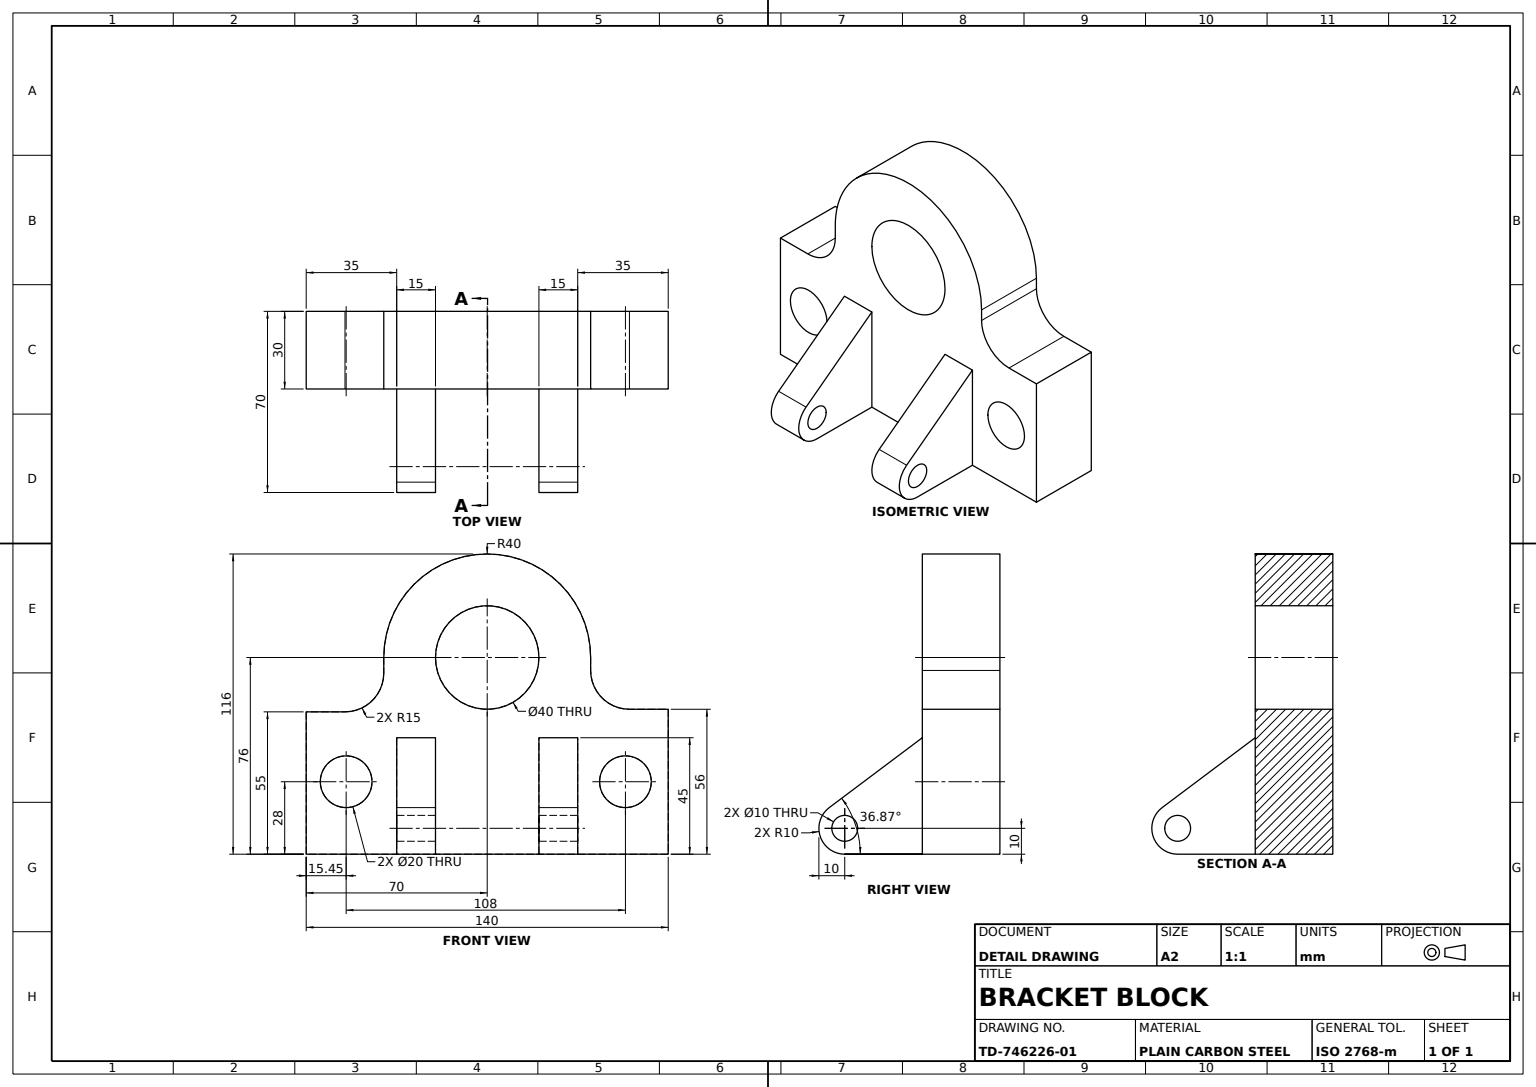
SolidWorks part; units mm, degrees
material "Plain Carbon Steel"
ref_plane "Front Plane" through (0, 0, 0) normal (0, 0, 1) x (1, 0, 0)
ref_plane "Top Plane" through (0, 0, 0) normal (0, 1, 0) x (1, 0, 0)
ref_plane "Right Plane" through (0, 0, 0) normal (1, 0, 0) x (0, 0, -1)
sketch "Base Plate Profile" plane through (0, 0, 0) normal (0, 0, 1) x (1, 0, 0)
  line L0 (0, 0) -> (140, 0)
  line L1 (140, 0) -> (140, 56)
  line L2 (0, 0) -> (0, 55)
  line L3 (0, 55) -> (15, 55)
  line L6 (140, 56) -> (125, 56)
  line L7 (30, 70) -> (30, 76)
  line L9 (110, 76) -> (110, 71)
  arc A0 (15, 55) -> (30, 70) centre (15, 70) ccw
  arc A1 (110, 71) -> (125, 56) centre (125, 71) ccw
  arc A2 (110, 76) -> (30, 76) centre (70, 76) ccw
  dimension "D1" = 140
  dimension "D2" = 71
  dimension "D3" = 76
  dimension "D5" = 15
  dimension "D6" = 40
  dimension "D4" = 76
  dimension "D7" = 55
extrude "Base Plate" add sketch "Base Plate Profile" along normal blind 30
sketch "Center Bore Profile" plane through (0, 0, 30) normal (0, 0, 1) x (1, 0, 0)
  circle A0 centre (70, 76) radius 20
  dimension "D1" = 40
extrude "Center Bore" cut sketch "Center Bore Profile" against normal blind 30
sketch "Side Holes Profile" plane through (0, 0, 30) normal (0, 0, 1) x (1, 0, 0)
  line L0 (0, 0) -> (140, 0) construction
  line L1 (0, 55) -> (0, 0) construction
  circle A0 centre (15.4516, 28) radius 10
  circle A1 centre (123.4516, 28) radius 10
  dimension "D1" = 28
  dimension "D4" = 20
  dimension "D2" = 28
  dimension "D3" = 108
  dimension "D5" = 15.4516
extrude "Side Holes 2xØ28" cut sketch "Side Holes Profile" against normal blind 30
sketch "Lug 1 Profile" plane through (0, 0, 0) normal (-1, 0, 0) x (0, 0, 1)
  line L0 (30, 0) -> (30, 45)
  line L1 (30, 55) -> (30, 0) construction
  line L2 (30, 0) -> (60, 0)
  line L3 (0, 55) -> (0, 0) construction
  line L4 (30, 45) -> (66, 18)
  arc A0 (60, 0) -> (66, 18) centre (60, 10) ccw
  dimension "D1" = 10
  dimension "D2" = 60
extrude "Lug 1" add sketch "Lug 1 Profile" against normal blind 50
sketch "Lug 1 Taper Profile" plane through (0, 0, 0) normal (-1, 0, 0) x (0, 0, 1)
  line L0 (30, 45) -> (30, 0)
  line L1 (60, 0) -> (0, 0) construction
  line L2 (30, 0) -> (60, 0)
  line L3 (30, 45) -> (66, 18)
  arc A0 (60, 0) -> (66, 18) centre (60, 10) ccw
extrude "Lug 1 Taper Cut" cut sketch "Lug 1 Taper Profile" against normal blind 35
sketch "Lug 1 Pin Hole Profile" plane through (35, 0, 0) normal (-1, 0, 0) x (0, 0, 1)
  circle A0 centre (60, 10) radius 5
  dimension "D1" = 10
extrude "Lug 1 Pin Hole" cut sketch "Lug 1 Pin Hole Profile" against normal blind 15
sketch "Lug 2 Profile" plane through (140, 0, 0) normal (1, 0, 0) x (0, 0, -1)
  line L0 (-30, 0) -> (-30, 45)
  line L1 (-30, 45) -> (-66, 18)
  line L2 (-30, 0) -> (-60, 0)
  arc A0 (-66, 18) -> (-60, 0) centre (-60, 10) ccw
extrude "Lug 2" add sketch "Lug 2 Profile" against normal blind 50
sketch "Lug 2 Taper Profile" plane through (140, 0, 0) normal (1, 0, 0) x (0, 0, -1)
  line L0 (-30, 45) -> (-66, 18)
  line L1 (-30, 45) -> (-30, 0)
  line L2 (-60, 0) -> (0, 0) construction
  line L3 (-30, 0) -> (-60, 0)
  arc A0 (-66, 18) -> (-60, 0) centre (-60, 10) ccw
extrude "Lug 2 Taper Cut" cut sketch "Lug 2 Taper Profile" against normal blind 35
sketch "Lug 2 Pin Hole Profile" plane through (105, 0, 0) normal (1, 0, 0) x (0, 0, -1)
  circle A0 centre (-60, 10) radius 5
  dimension "D1" = 10
extrude "Lug 2 Pin Hole" cut sketch "Lug 2 Pin Hole Profile" against normal blind 15
